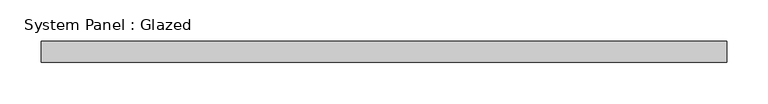
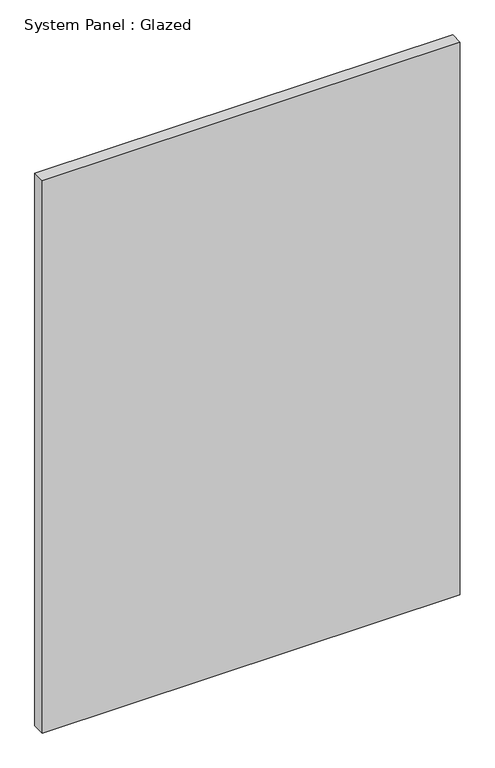
"""IFC4 building model written with IfcOpenShell, lengths in millimetres: plate geometry, System Panel : Glazed."""

from ifc_helpers import new_model, si_unit, origin, origin_with_axes, place, context, project, spatial, polyline, outline, extrude, source, transform, mapped, element, save


def system_panel_glazed_fc8e0588(model_context):
    return source(origin(), model_context, "Body", "SweptSolid", [
        extrude(outline(polyline([(413.7856373, 19.05), (-413.7856373, 19.05), (-413.7856373, 44.45), (413.7856373, 44.45), (413.7856373, 19.05)])), origin_with_axes(), (0.0, 0.0, 1.0), 1155.7),
    ])


if __name__ == "__main__":
    model = new_model("IFC4")
    model_context = context("Model", 3, world=origin())
    ifc_project = project(units=[si_unit("LENGTHUNIT", "METRE", prefix="MILLI")], contexts=[model_context])
    site = spatial("IfcSite", under=ifc_project)
    building = spatial("IfcBuilding", under=site)
    placement = place(None, origin())
    system_panel_glazed_shape = system_panel_glazed_fc8e0588(model_context)
    element("IfcPlate", 1, ObjectType="System Panel : Glazed", at=placement, inside=building, context=model_context, shape_type="MappedRepresentation", body=[
        mapped(system_panel_glazed_shape, transform((0.0, 0.0, 0.0), x_axis=(1.0, 0.0, 0.0), y_axis=(0.0, 1.0, 0.0), z_axis=(0.0, 0.0, 1.0))),
    ])
    save(model, "model.ifc")

# Revit data of these elements
# Type "System Panel : Glazed"
#   Construction Type Id = "GSP4R"
#   Analytic Construction = "1/8 in Pilkington single glazing"
#   Visual Light Transmittance = 0.9
#   Solar Heat Gain Coefficient = 0.86
#   Heat Transfer Coefficient (U) = 1.18115 BTU/(h·ft²·°F)
# Element 1 (IfcPlate, "System Panel : Glazed")
#   Materials on its faces: "Glass"
# Materials
#   "Glass": class "Glass", colour RGB 0 128 192, transparency 0.75, Description = "Soda Lime Glass", Cost = 0
